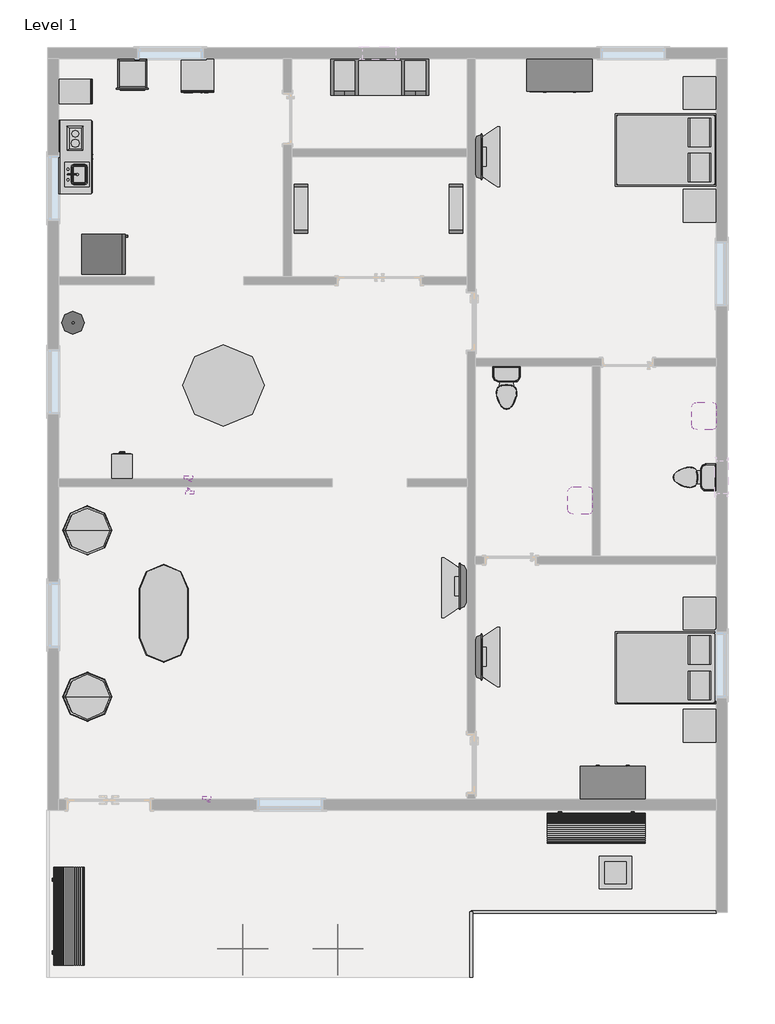
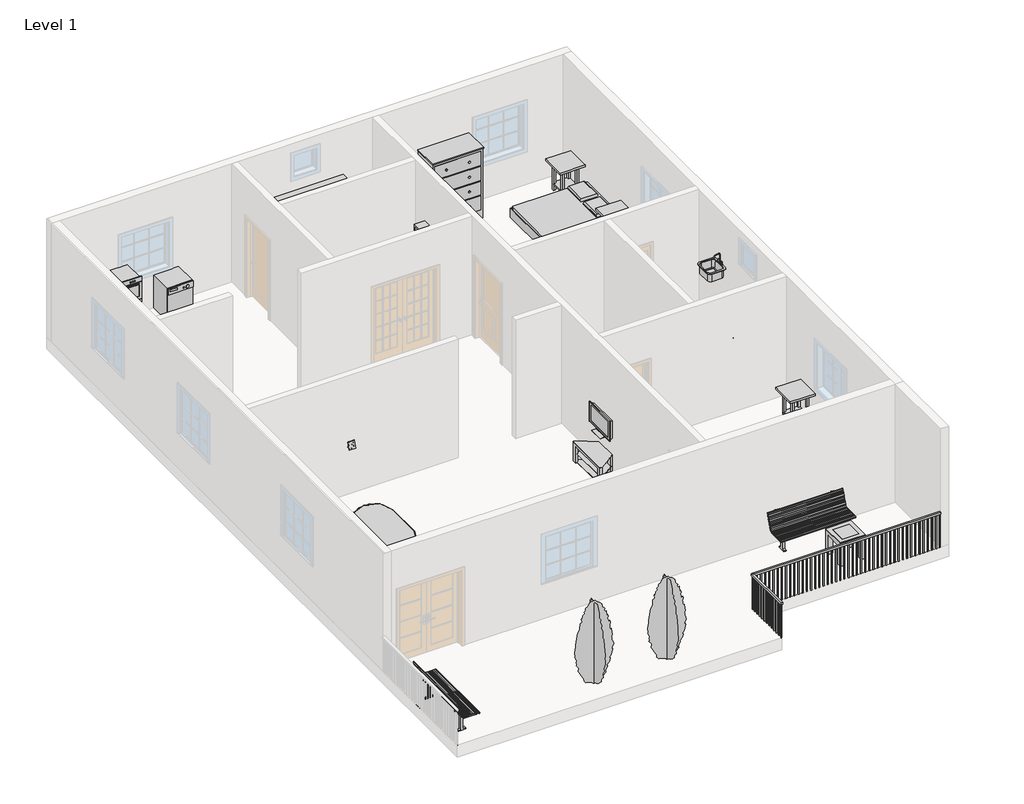
# One storey, part 2 of 2: 24 furniture elements, 11 proxies, 6 flow terminals, 4 geographic elements, 2 railings.
"""IFC4 building model written with IfcOpenShell, lengths in millimetres."""

from ifc_helpers import new_model, si_unit, frame, origin, origin_with_axes, place, context, project, spatial, polyline, outline, extrude, triangles, transform, mapped, element, save
from components import proxy_7e1014cc, proxy_fe84b772, proxy_45b28599, proxy_844211aa, proxy_8b8c2dc4, rpc_picture_frame_rpc_picture_frame_c25e3fe9, proxy_a13a33b2, flow_terminal_871c2e40, flow_terminal_d49f872f, flow_terminal_62a433f7, toilet_domestic_3d_toilet_domestic_3d_f7549cf7, toilet_domestic_3d_toilet_domestic_3d_183bbd19, furniture_c8abb964, furniture_552c1472, furniture_95afb093, furniture_9fa109b2, furniture_cf0b6580, furniture_417d203a, furniture_56245f3a, tv_stand_tv_stand_6ce107e5, furniture_b5c51a22, furniture_2c34a4f9, furniture_bbcc68ce, furniture_5bc9ed15, furniture_c80d6d9c, geographic_element_235d1464, rpc_tree_conifer_chinese_juniper_7_1b9786cd

model = new_model("IFC4")

# Units and contexts
model_context = context("Model", 3, world=origin())
ifc_project = project(units=[si_unit("LENGTHUNIT", "METRE", prefix="MILLI")], contexts=[model_context])

# Site, building, storey
site = spatial("IfcSite", under=ifc_project)
building = spatial("IfcBuilding", under=site)
storey = spatial("IfcBuildingStorey", under=building, Name="Level 1", Elevation=0.0)

# Proxies
placement = place(None, origin())
element("IfcBuildingElementProxy", 1, Name="Building Element Proxy", at=placement, inside=storey, context=model_context, shape_type="Tessellation", body=[
    triangles([(-15555.8644409, -380.8198874, 0.0), (-15555.8644409, -3505.0197784, 0.0), (-7656.4646347, -3505.0197784, 0.0), (-7656.4646347, -2285.8199238, 0.0), (-7647.9977097, -380.8198874, 0.0)], [[1, 2, 4], [4, 3, 5], [3, 4, 2], [4, 5, 1]], closed=False),
])
element("IfcBuildingElementProxy", 2, Name="Building Element Proxy", at=placement, inside=storey, context=model_context, shape_type="Tessellation", body=[
    triangles([(-7656.4646347, -2285.8199238, 0.0), (-3084.4649254, -2285.8199238, 0.0), (-3084.4649254, -380.8198874, 0.0), (-7643.7130875, -380.8198874, 0.0), (-7647.8139999, -380.8198874, 0.0)], [[5, 1, 4], [4, 2, 3], [2, 4, 1]], closed=False),
])
proxy_shape = proxy_7e1014cc(model_context)
element("IfcBuildingElementProxy", 3, Name="18\" x 24\" x 34 1/2\"", ObjectType="18\" x 24\" x 34 1/2\"", at=placement, inside=storey, context=model_context, shape_type="MappedRepresentation", body=[
    mapped(proxy_shape, transform((-14781.4152961, 12724.2626366, 0.0), x_axis=(0.0, 1.0, 0.0), y_axis=(-1.0, 0.0, 0.0), z_axis=(0.0, 0.0, 1.0))),
])
proxy_2_shape = proxy_fe84b772(model_context)
element("IfcBuildingElementProxy", 4, Name="Cook Top-2 Unit : 12\" x 18\"", ObjectType="Cook Top-2 Unit : 12\" x 18\"", at=placement, inside=storey, context=model_context, shape_type="MappedRepresentation", body=[
    mapped(proxy_2_shape, transform((-14971.6648609, 12184.3049007, 0.0), x_axis=(-1.0, 0.0, 0.0), y_axis=(0.0, -1.0, 0.0), z_axis=(0.0, 0.0, 1.0))),
])
proxy_3_shape = proxy_45b28599(model_context)
element("IfcBuildingElementProxy", 5, Name="Dishwasher : 24\" x 24\" x 34\"", ObjectType="Dishwasher : 24\" x 24\" x 34\"", at=placement, inside=storey, context=model_context, shape_type="MappedRepresentation", body=[
    mapped(proxy_3_shape, transform((-13144.1823294, 13068.7305403, 0.0), x_axis=(1.0, 0.0, 0.0), y_axis=(0.0, 1.0, 0.0), z_axis=(0.0, 0.0, 1.0))),
])
proxy_4_shape = proxy_844211aa(model_context)
element("IfcBuildingElementProxy", 6, Name="Kitchenette - Small : 54\"", ObjectType="Kitchenette - Small : 54\"", at=placement, inside=storey, context=model_context, shape_type="MappedRepresentation", body=[
    mapped(proxy_4_shape, transform((-15352.6648609, 11792.4424002, 0.0), x_axis=(0.0, 1.0, 0.0), y_axis=(-1.0, 0.0, 0.0), z_axis=(0.0, 0.0, 1.0))),
])
proxy_5_shape = proxy_8b8c2dc4(model_context)
element("IfcBuildingElementProxy", 7, Name="Oven Double-Built-in : 21 1/2\" x 39 1/4\" x 21\"", ObjectType="Oven Double-Built-in : 21 1/2\" x 39 1/4\" x 21\"", at=placement, inside=storey, context=model_context, shape_type="MappedRepresentation", body=[
    mapped(proxy_5_shape, transform((-13945.8899336, 13219.5142461, 0.0), x_axis=(1.0, 0.0, 0.0), y_axis=(0.0, 1.0, 0.0), z_axis=(0.0, 0.0, 1.0))),
])
rpc_picture_frame_rpc_picture_frame_shape = rpc_picture_frame_rpc_picture_frame_c25e3fe9(model_context)
element("IfcBuildingElementProxy", 8, Name="RPC Picture Frame : RPC Picture Frame", ObjectType="RPC Picture Frame : RPC Picture Frame", at=placement, inside=storey, context=model_context, shape_type="MappedRepresentation", body=[
    mapped(rpc_picture_frame_rpc_picture_frame_shape, transform((-12906.6432707, 5575.4801051, 1219.2), x_axis=(1.0, 0.0, 0.0), y_axis=(0.0, 1.0, 0.0), z_axis=(0.0, 0.0, 1.0))),
])
element("IfcBuildingElementProxy", 9, Name="RPC Picture Frame : RPC Picture Frame", ObjectType="RPC Picture Frame : RPC Picture Frame", at=placement, inside=storey, context=model_context, shape_type="MappedRepresentation", body=[
    mapped(rpc_picture_frame_rpc_picture_frame_shape, transform((-12590.3070473, -177.6198949, 1219.2), x_axis=(-1.0000000000000004, 0.0, 0.0), y_axis=(0.0, -1.0000000000000004, 0.0), z_axis=(0.0, 0.0, 1.0))),
])
element("IfcBuildingElementProxy", 10, Name="RPC Picture Frame : RPC Picture Frame", ObjectType="RPC Picture Frame : RPC Picture Frame", at=placement, inside=storey, context=model_context, shape_type="MappedRepresentation", body=[
    mapped(rpc_picture_frame_rpc_picture_frame_shape, transform((-12931.6137427, 5804.0801051, 1219.2), x_axis=(-1.0, 0.0, 0.0), y_axis=(0.0, -1.0, 0.0), z_axis=(0.0, 0.0, 1.0))),
])
proxy_6_shape = proxy_a13a33b2(model_context)
element("IfcBuildingElementProxy", 11, Name="Refrigerator : 30\" x 32\" RH", ObjectType="Refrigerator : 30\" x 32\" RH", at=placement, inside=storey, context=model_context, shape_type="MappedRepresentation", body=[
    mapped(proxy_6_shape, transform((-14531.9273609, 9993.8811336, 0.0), x_axis=(0.0, 1.000000000000001, 0.0), y_axis=(-1.000000000000001, 0.0, 0.0), z_axis=(0.0, 0.0, 1.0))),
])

# Flow terminals
flow_terminal_shape = flow_terminal_871c2e40(model_context)
element("IfcFlowTerminal", 12, ObjectType="Sink Kitchen-Island : 18\" x 18\"", at=placement, inside=storey, context=model_context, shape_type="MappedRepresentation", body=[
    mapped(flow_terminal_shape, transform((-15007.4194598, 11465.2908645, 0.0), x_axis=(0.0, 1.0, 0.0), y_axis=(-1.0, 0.0, 0.0), z_axis=(0.0, 0.0, 1.0))),
])
flow_terminal_2_shape = flow_terminal_d49f872f(model_context)
element("IfcFlowTerminal", 13, ObjectType="Sink Vanity-Round : 19\" x 19\"", at=placement, inside=storey, context=model_context, shape_type="MappedRepresentation", body=[
    mapped(flow_terminal_2_shape, transform((-15003.148195, 8615.7283645, 609.6), x_axis=(0.0, 1.0000000000000009, 0.0), y_axis=(-1.0000000000000009, 0.0, 0.0), z_axis=(0.0, 0.0, 1.0))),
])
flow_terminal_3_shape = flow_terminal_62a433f7(model_context)
element("IfcFlowTerminal", 14, ObjectType="Sink Vanity-Square : 20\" x 18\"", at=placement, inside=storey, context=model_context, shape_type="MappedRepresentation", body=[
    mapped(flow_terminal_3_shape, transform((-3264.610262, 6988.1693456, 914.4), x_axis=(0.0, -1.0, 0.0), y_axis=(1.0, 0.0, 0.0), z_axis=(0.0, 0.0, 1.0))),
])
element("IfcFlowTerminal", 15, ObjectType="Sink Vanity-Square : 20\" x 18\"", at=placement, inside=storey, context=model_context, shape_type="MappedRepresentation", body=[
    mapped(flow_terminal_3_shape, transform((-5576.010262, 5413.3693456, 914.4), x_axis=(0.0, -1.0000000000000002, 0.0), y_axis=(1.0000000000000002, 0.0, 0.0), z_axis=(0.0, 0.0, 1.0))),
])
toilet_domestic_3d_toilet_domestic_3d_shape = toilet_domestic_3d_toilet_domestic_3d_f7549cf7(model_context)
toilet_domestic_3d_toilet_domestic_3d_2_shape = toilet_domestic_3d_toilet_domestic_3d_183bbd19(model_context)
element("IfcFlowTerminal", 16, ObjectType="Toilet-Domestic-3D : Toilet-Domestic-3D", at=placement, inside=storey, context=model_context, shape_type="MappedRepresentation", body=[
    mapped(toilet_domestic_3d_toilet_domestic_3d_shape, transform((-6996.0648609, 7404.8840777, 0.0), x_axis=(1.0, 0.0, 0.0), y_axis=(0.0, 1.0, 0.0), z_axis=(0.0, 0.0, 1.0))),
    mapped(toilet_domestic_3d_toilet_domestic_3d_2_shape, transform((-6996.0648609, 7404.8840777, 0.0), x_axis=(1.0, 0.0, 0.0), y_axis=(0.0, 1.0, 0.0), z_axis=(0.0, 0.0, 1.0))),
])
element("IfcFlowTerminal", 17, ObjectType="Toilet-Domestic-3D : Toilet-Domestic-3D", at=placement, inside=storey, context=model_context, shape_type="MappedRepresentation", body=[
    mapped(toilet_domestic_3d_toilet_domestic_3d_shape, transform((-3579.1608883, 5829.4801051, 0.0), x_axis=(0.0, -1.0000000000000007, 0.0), y_axis=(1.0000000000000007, 0.0, 0.0), z_axis=(0.0, 0.0, 1.0))),
    mapped(toilet_domestic_3d_toilet_domestic_3d_2_shape, transform((-3579.1608883, 5829.4801051, 0.0), x_axis=(0.0, -1.0000000000000007, 0.0), y_axis=(1.0000000000000007, 0.0, 0.0), z_axis=(0.0, 0.0, 1.0))),
])

# Furniture
furniture_shape = furniture_c8abb964(model_context)
element("IfcFurniture", 18, ObjectType="Bed-Box : Double 53\" x 74\"", at=placement, inside=storey, context=model_context, shape_type="MappedRepresentation", body=[
    mapped(furniture_shape, transform((-3789.8353527, 2612.6325641, 0.0), x_axis=(0.0, -1.0, 0.0), y_axis=(1.0, 0.0, 0.0), z_axis=(0.0, 0.0, 1.0))),
])
element("IfcFurniture", 19, ObjectType="Bed-Box : Double 53\" x 74\"", at=placement, inside=storey, context=model_context, shape_type="MappedRepresentation", body=[
    mapped(furniture_shape, transform((-3789.8353527, 12277.3325641, 0.0), x_axis=(0.0, -1.0, 0.0), y_axis=(1.0, 0.0, 0.0), z_axis=(0.0, 0.0, 1.0))),
])
furniture_2_shape = furniture_552c1472(model_context)
element("IfcFurniture", 20, ObjectType="Cabinet-File 3 Drawer : 15\" x 18\"", at=placement, inside=storey, context=model_context, shape_type="MappedRepresentation", body=[
    mapped(furniture_2_shape, transform((-14299.4613079, 5890.545805, 0.0), x_axis=(-1.0, 0.0, 0.0), y_axis=(0.0, -1.0, 0.0), z_axis=(0.0, 0.0, 1.0))),
])
furniture_3_shape = furniture_95afb093(model_context)
element("IfcFurniture", 21, ObjectType="Counter Top w Sink Hole : 24\" Depth", at=placement, inside=storey, context=model_context, shape_type="MappedRepresentation", body=[
    mapped(furniture_3_shape, transform((-15352.6648609, 12325.8424002, 0.0), x_axis=(0.0, 1.0, 0.0), y_axis=(-1.0, 0.0, 0.0), z_axis=(0.0, 0.0, 1.0))),
])
furniture_4_shape = furniture_9fa109b2(model_context)
element("IfcFurniture", 22, ObjectType="Dresser : 48\" x 72\" x 24\"", at=placement, inside=storey, context=model_context, shape_type="MappedRepresentation", body=[
    mapped(furniture_4_shape, transform((-5284.0581207, -235.982849, 0.0), x_axis=(-1.0000000000000004, 0.0, 0.0), y_axis=(0.0, -1.0000000000000004, 0.0), z_axis=(0.0, 0.0, 1.0))),
])
element("IfcFurniture", 23, ObjectType="Dresser : 48\" x 72\" x 24\"", at=placement, inside=storey, context=model_context, shape_type="MappedRepresentation", body=[
    mapped(furniture_4_shape, transform((-5736.2716011, 13698.3430592, 0.0), x_axis=(1.0, 0.0, 0.0), y_axis=(0.0, 1.0, 0.0), z_axis=(0.0, 0.0, 1.0))),
])
furniture_5_shape = furniture_cf0b6580(model_context)
element("IfcFurniture", 24, ObjectType="Entertainment Center : 72\" x 72\" x 24\"", at=placement, inside=storey, context=model_context, shape_type="MappedRepresentation", body=[
    mapped(furniture_5_shape, transform((-9358.2648609, 13741.5801051, 0.0), x_axis=(1.0, 0.0, 0.0), y_axis=(0.0, 1.0, 0.0), z_axis=(0.0, 0.0, 1.0))),
])
furniture_6_shape = furniture_417d203a(model_context)
element("IfcFurniture", 25, ObjectType="Shelving : 36\" x 10\" x 72\"", at=placement, inside=storey, context=model_context, shape_type="MappedRepresentation", body=[
    mapped(furniture_6_shape, transform((-11136.2648609, 10845.9801051, 0.0), x_axis=(0.0, 1.0000000000000002, 0.0), y_axis=(-1.0000000000000002, 0.0, 0.0), z_axis=(0.0, 0.0, 1.0))),
])
element("IfcFurniture", 26, ObjectType="Shelving : 36\" x 10\" x 72\"", at=placement, inside=storey, context=model_context, shape_type="MappedRepresentation", body=[
    mapped(furniture_6_shape, transform((-8240.6648609, 10845.9801051, 0.0), x_axis=(0.0, 1.0000000000000002, 0.0), y_axis=(-1.0000000000000002, 0.0, 0.0), z_axis=(0.0, 0.0, 1.0))),
])
furniture_7_shape = furniture_56245f3a(model_context)
element("IfcFurniture", 27, ObjectType="TV - Flat Screen : 32\"", at=placement, inside=storey, context=model_context, shape_type="MappedRepresentation", body=[
    mapped(furniture_7_shape, transform((-7521.7262373, 2480.6246192, 914.4), x_axis=(0.0, 1.0000000000000002, 0.0), y_axis=(-1.0000000000000002, 0.0, 0.0), z_axis=(0.0, 0.0, 1.0))),
])
element("IfcFurniture", 28, ObjectType="TV - Flat Screen : 32\"", at=placement, inside=storey, context=model_context, shape_type="MappedRepresentation", body=[
    mapped(furniture_7_shape, transform((-7521.7262373, 11815.1246192, 914.4), x_axis=(0.0, 1.0000000000000002, 0.0), y_axis=(-1.0000000000000002, 0.0, 0.0), z_axis=(0.0, 0.0, 1.0))),
])
element("IfcFurniture", 29, ObjectType="TV - Flat Screen : 32\"", at=placement, inside=storey, context=model_context, shape_type="MappedRepresentation", body=[
    mapped(furniture_7_shape, transform((-7810.4777417, 3791.9647442, 914.4), x_axis=(0.0, -1.0000000000000007, 0.0), y_axis=(1.0000000000000007, 0.0, 0.0), z_axis=(0.0, 0.0, 1.0))),
])
tv_stand_tv_stand_shape = tv_stand_tv_stand_6ce107e5(model_context)
element("IfcFurniture", 30, ObjectType="TV Stand : TV Stand", at=placement, inside=storey, context=model_context, shape_type="MappedRepresentation", body=[
    mapped(tv_stand_tv_stand_shape, transform((-7580.2648609, 11685.992103, 0.0), x_axis=(0.0, 1.0000000000000002, 0.0), y_axis=(-1.0000000000000002, 0.0, 0.0), z_axis=(0.0, 0.0, 1.0))),
])
element("IfcFurniture", 31, ObjectType="TV Stand : TV Stand", at=placement, inside=storey, context=model_context, shape_type="MappedRepresentation", body=[
    mapped(tv_stand_tv_stand_shape, transform((-7580.2648609, 2351.492103, 0.0), x_axis=(0.0, 1.0000000000000002, 0.0), y_axis=(-1.0000000000000002, 0.0, 0.0), z_axis=(0.0, 0.0, 1.0))),
])
element("IfcFurniture", 32, ObjectType="TV Stand : TV Stand", at=placement, inside=storey, context=model_context, shape_type="MappedRepresentation", body=[
    mapped(tv_stand_tv_stand_shape, transform((-7747.8095547, 3895.3169532, 0.0), x_axis=(0.0, -1.0000000000000007, 0.0), y_axis=(1.0000000000000007, 0.0, 0.0), z_axis=(0.0, 0.0, 1.0))),
])
furniture_8_shape = furniture_b5c51a22(model_context)
element("IfcFurniture", 33, ObjectType="Table-Coffee : 24\" x 24\" x 24\"", at=placement, inside=storey, context=model_context, shape_type="MappedRepresentation", body=[
    mapped(furniture_8_shape, transform((-4982.3306276, -1644.4309727, 0.0), x_axis=(1.0, 0.0, 0.0), y_axis=(0.0, 1.0, 0.0), z_axis=(0.0, 0.0, 1.0))),
])
furniture_9_shape = furniture_2c34a4f9(model_context)
element("IfcFurniture", 34, ObjectType="Table-Dining Oval : 36\" x 72\"", at=placement, inside=storey, context=model_context, shape_type="MappedRepresentation", body=[
    mapped(furniture_9_shape, transform((-13754.9632216, 3691.2997772, 0.0), x_axis=(0.0, 1.0000000000000002, 0.0), y_axis=(-1.0000000000000002, 0.0, 0.0), z_axis=(0.0, 0.0, 1.0))),
])
furniture_10_shape = furniture_bbcc68ce(model_context)
element("IfcFurniture", 35, ObjectType="Table-Dining Round w Chairs : 60\" Diameter", at=placement, inside=storey, context=model_context, shape_type="MappedRepresentation", body=[
    mapped(furniture_10_shape, transform((-12382.9468281, 7728.8587936, 0.0), x_axis=(1.0, 0.0, 0.0), y_axis=(0.0, 1.0, 0.0), z_axis=(0.0, 0.0, 1.0))),
])
furniture_11_shape = furniture_5bc9ed15(model_context)
element("IfcFurniture", 36, ObjectType="Table-Night Stand : 24\" x 24\" x 30\"", at=placement, inside=storey, context=model_context, shape_type="MappedRepresentation", body=[
    mapped(furniture_11_shape, transform((-3697.7984912, 2984.6801051, 0.0), x_axis=(1.0, 0.0, 0.0), y_axis=(0.0, 1.0, 0.0), z_axis=(0.0, 0.0, 1.0))),
])
element("IfcFurniture", 37, ObjectType="Table-Night Stand : 24\" x 24\" x 30\"", at=placement, inside=storey, context=model_context, shape_type="MappedRepresentation", body=[
    mapped(furniture_11_shape, transform((-3697.7984912, 889.1801051, 0.0), x_axis=(1.0, 0.0, 0.0), y_axis=(0.0, 1.0, 0.0), z_axis=(0.0, 0.0, 1.0))),
])
element("IfcFurniture", 38, ObjectType="Table-Night Stand : 24\" x 24\" x 30\"", at=placement, inside=storey, context=model_context, shape_type="MappedRepresentation", body=[
    mapped(furniture_11_shape, transform((-3697.7984912, 12700.1801051, 0.0), x_axis=(1.0, 0.0, 0.0), y_axis=(0.0, 1.0, 0.0), z_axis=(0.0, 0.0, 1.0))),
])
element("IfcFurniture", 39, ObjectType="Table-Night Stand : 24\" x 24\" x 30\"", at=placement, inside=storey, context=model_context, shape_type="MappedRepresentation", body=[
    mapped(furniture_11_shape, transform((-3697.7984912, 10591.9801051, 0.0), x_axis=(1.0, 0.0, 0.0), y_axis=(0.0, 1.0, 0.0), z_axis=(0.0, 0.0, 1.0))),
])
furniture_12_shape = furniture_c80d6d9c(model_context)
element("IfcFurniture", 40, ObjectType="Table-Round : 36\" Diameter", at=placement, inside=storey, context=model_context, shape_type="MappedRepresentation", body=[
    mapped(furniture_12_shape, transform((-14819.2648609, 4838.8801051, 0.0), x_axis=(1.0, 0.0, 0.0), y_axis=(0.0, 1.0, 0.0), z_axis=(0.0, 0.0, 1.0))),
])
element("IfcFurniture", 41, ObjectType="Table-Round : 36\" Diameter", at=placement, inside=storey, context=model_context, shape_type="MappedRepresentation", body=[
    mapped(furniture_12_shape, transform((-14819.2648609, 1733.7301051, 0.0), x_axis=(1.0, 0.0, 0.0), y_axis=(0.0, 1.0, 0.0), z_axis=(0.0, 0.0, 1.0))),
])

# Geographic elements
geographic_element_shape = geographic_element_235d1464(model_context)
element("IfcGeographicElement", 42, ObjectType="Park Bench : 72\"", at=placement, inside=storey, context=model_context, shape_type="MappedRepresentation", body=[
    mapped(geographic_element_shape, transform((-15200.2648609, -2362.0198949, 0.0), x_axis=(0.0, 1.0000000000000002, 0.0), y_axis=(-1.0000000000000002, 0.0, 0.0), z_axis=(0.0, 0.0, 1.0))),
])
element("IfcGeographicElement", 43, ObjectType="Park Bench : 72\"", at=placement, inside=storey, context=model_context, shape_type="MappedRepresentation", body=[
    mapped(geographic_element_shape, transform((-5319.6648609, -685.6198949, 0.0), x_axis=(1.0, 0.0, 0.0), y_axis=(0.0, 1.0, 0.0), z_axis=(0.0, 0.0, 1.0))),
])
rpc_tree_conifer_chinese_juniper_7_shape = rpc_tree_conifer_chinese_juniper_7_1b9786cd(model_context)
element("IfcGeographicElement", 44, ObjectType="RPC Tree - Conifer : Chinese Juniper - 7'", at=placement, inside=storey, context=model_context, shape_type="MappedRepresentation", body=[
    mapped(rpc_tree_conifer_chinese_juniper_7_shape, transform((-11923.861532, -2971.6198949, 0.0), x_axis=(1.0, 0.0, 0.0), y_axis=(0.0, 1.0, 0.0), z_axis=(0.0, 0.0, 1.0))),
])
element("IfcGeographicElement", 45, ObjectType="RPC Tree - Conifer : Chinese Juniper - 7'", at=placement, inside=storey, context=model_context, shape_type="MappedRepresentation", body=[
    mapped(rpc_tree_conifer_chinese_juniper_7_shape, transform((-10145.861532, -2971.6198949, 0.0), x_axis=(1.0, 0.0, 0.0), y_axis=(0.0, 1.0, 0.0), z_axis=(0.0, 0.0, 1.0))),
])

# Railings
element("IfcRailing", 46, ObjectType="Handrail - Rectangular", at=placement, inside=storey, context=model_context, shape_type="SweptSolid", body=[
    extrude(outline(polyline([(-3084.4648609, -2260.4198949), (-3084.4648609, -2311.2198949), (-7656.4648609, -2311.2198949), (-7656.4648609, -2260.4198949), (-3084.4648609, -2260.4198949)])), frame((0.0, 0.0, 863.6), z_axis=(0.0, 0.0, 1.0), x_axis=(1.0, 0.0, 0.0)), (0.0, 0.0, 1.0), 50.8),
    extrude(outline(polyline([(-7545.3398609, -2276.2948949), (-7545.3398609, -2295.3448949), (-7564.3898609, -2295.3448949), (-7564.3898609, -2276.2948949), (-7545.3398609, -2276.2948949)])), origin_with_axes(), (0.0, 0.0, 1.0), 863.6),
    extrude(outline(polyline([(-7443.7398609, -2276.2948949), (-7443.7398609, -2295.3448949), (-7462.7898609, -2295.3448949), (-7462.7898609, -2276.2948949), (-7443.7398609, -2276.2948949)])), origin_with_axes(), (0.0, 0.0, 1.0), 863.6),
    extrude(outline(polyline([(-7342.1398609, -2276.2948949), (-7342.1398609, -2295.3448949), (-7361.1898609, -2295.3448949), (-7361.1898609, -2276.2948949), (-7342.1398609, -2276.2948949)])), origin_with_axes(), (0.0, 0.0, 1.0), 863.6),
    extrude(outline(polyline([(-7240.5398609, -2276.2948949), (-7240.5398609, -2295.3448949), (-7259.5898609, -2295.3448949), (-7259.5898609, -2276.2948949), (-7240.5398609, -2276.2948949)])), origin_with_axes(), (0.0, 0.0, 1.0), 863.6),
    extrude(outline(polyline([(-7138.9398609, -2276.2948949), (-7138.9398609, -2295.3448949), (-7157.9898609, -2295.3448949), (-7157.9898609, -2276.2948949), (-7138.9398609, -2276.2948949)])), origin_with_axes(), (0.0, 0.0, 1.0), 863.6),
    extrude(outline(polyline([(-7037.3398609, -2276.2948949), (-7037.3398609, -2295.3448949), (-7056.3898609, -2295.3448949), (-7056.3898609, -2276.2948949), (-7037.3398609, -2276.2948949)])), origin_with_axes(), (0.0, 0.0, 1.0), 863.6),
    extrude(outline(polyline([(-6935.7398609, -2276.2948949), (-6935.7398609, -2295.3448949), (-6954.7898609, -2295.3448949), (-6954.7898609, -2276.2948949), (-6935.7398609, -2276.2948949)])), origin_with_axes(), (0.0, 0.0, 1.0), 863.6),
    extrude(outline(polyline([(-6834.1398609, -2276.2948949), (-6834.1398609, -2295.3448949), (-6853.1898609, -2295.3448949), (-6853.1898609, -2276.2948949), (-6834.1398609, -2276.2948949)])), origin_with_axes(), (0.0, 0.0, 1.0), 863.6),
    extrude(outline(polyline([(-6732.5398609, -2276.2948949), (-6732.5398609, -2295.3448949), (-6751.5898609, -2295.3448949), (-6751.5898609, -2276.2948949), (-6732.5398609, -2276.2948949)])), origin_with_axes(), (0.0, 0.0, 1.0), 863.6),
    extrude(outline(polyline([(-6630.9398609, -2276.2948949), (-6630.9398609, -2295.3448949), (-6649.9898609, -2295.3448949), (-6649.9898609, -2276.2948949), (-6630.9398609, -2276.2948949)])), origin_with_axes(), (0.0, 0.0, 1.0), 863.6),
    extrude(outline(polyline([(-6529.3398609, -2276.2948949), (-6529.3398609, -2295.3448949), (-6548.3898609, -2295.3448949), (-6548.3898609, -2276.2948949), (-6529.3398609, -2276.2948949)])), origin_with_axes(), (0.0, 0.0, 1.0), 863.6),
    extrude(outline(polyline([(-6427.7398609, -2276.2948949), (-6427.7398609, -2295.3448949), (-6446.7898609, -2295.3448949), (-6446.7898609, -2276.2948949), (-6427.7398609, -2276.2948949)])), origin_with_axes(), (0.0, 0.0, 1.0), 863.6),
    extrude(outline(polyline([(-6326.1398609, -2276.2948949), (-6326.1398609, -2295.3448949), (-6345.1898609, -2295.3448949), (-6345.1898609, -2276.2948949), (-6326.1398609, -2276.2948949)])), origin_with_axes(), (0.0, 0.0, 1.0), 863.6),
    extrude(outline(polyline([(-6224.5398609, -2276.2948949), (-6224.5398609, -2295.3448949), (-6243.5898609, -2295.3448949), (-6243.5898609, -2276.2948949), (-6224.5398609, -2276.2948949)])), origin_with_axes(), (0.0, 0.0, 1.0), 863.6),
    extrude(outline(polyline([(-6122.9398609, -2276.2948949), (-6122.9398609, -2295.3448949), (-6141.9898609, -2295.3448949), (-6141.9898609, -2276.2948949), (-6122.9398609, -2276.2948949)])), origin_with_axes(), (0.0, 0.0, 1.0), 863.6),
    extrude(outline(polyline([(-6021.3398609, -2276.2948949), (-6021.3398609, -2295.3448949), (-6040.3898609, -2295.3448949), (-6040.3898609, -2276.2948949), (-6021.3398609, -2276.2948949)])), origin_with_axes(), (0.0, 0.0, 1.0), 863.6),
    extrude(outline(polyline([(-5919.7398609, -2276.2948949), (-5919.7398609, -2295.3448949), (-5938.7898609, -2295.3448949), (-5938.7898609, -2276.2948949), (-5919.7398609, -2276.2948949)])), origin_with_axes(), (0.0, 0.0, 1.0), 863.6),
    extrude(outline(polyline([(-5818.1398609, -2276.2948949), (-5818.1398609, -2295.3448949), (-5837.1898609, -2295.3448949), (-5837.1898609, -2276.2948949), (-5818.1398609, -2276.2948949)])), origin_with_axes(), (0.0, 0.0, 1.0), 863.6),
    extrude(outline(polyline([(-5716.5398609, -2276.2948949), (-5716.5398609, -2295.3448949), (-5735.5898609, -2295.3448949), (-5735.5898609, -2276.2948949), (-5716.5398609, -2276.2948949)])), origin_with_axes(), (0.0, 0.0, 1.0), 863.6),
    extrude(outline(polyline([(-5614.9398609, -2276.2948949), (-5614.9398609, -2295.3448949), (-5633.9898609, -2295.3448949), (-5633.9898609, -2276.2948949), (-5614.9398609, -2276.2948949)])), origin_with_axes(), (0.0, 0.0, 1.0), 863.6),
    extrude(outline(polyline([(-5513.3398609, -2276.2948949), (-5513.3398609, -2295.3448949), (-5532.3898609, -2295.3448949), (-5532.3898609, -2276.2948949), (-5513.3398609, -2276.2948949)])), origin_with_axes(), (0.0, 0.0, 1.0), 863.6),
    extrude(outline(polyline([(-5411.7398609, -2276.2948949), (-5411.7398609, -2295.3448949), (-5430.7898609, -2295.3448949), (-5430.7898609, -2276.2948949), (-5411.7398609, -2276.2948949)])), origin_with_axes(), (0.0, 0.0, 1.0), 863.6),
    extrude(outline(polyline([(-5310.1398609, -2276.2948949), (-5310.1398609, -2295.3448949), (-5329.1898609, -2295.3448949), (-5329.1898609, -2276.2948949), (-5310.1398609, -2276.2948949)])), origin_with_axes(), (0.0, 0.0, 1.0), 863.6),
    extrude(outline(polyline([(-5208.5398609, -2276.2948949), (-5208.5398609, -2295.3448949), (-5227.5898609, -2295.3448949), (-5227.5898609, -2276.2948949), (-5208.5398609, -2276.2948949)])), origin_with_axes(), (0.0, 0.0, 1.0), 863.6),
    extrude(outline(polyline([(-5106.9398609, -2276.2948949), (-5106.9398609, -2295.3448949), (-5125.9898609, -2295.3448949), (-5125.9898609, -2276.2948949), (-5106.9398609, -2276.2948949)])), origin_with_axes(), (0.0, 0.0, 1.0), 863.6),
    extrude(outline(polyline([(-5005.3398609, -2276.2948949), (-5005.3398609, -2295.3448949), (-5024.3898609, -2295.3448949), (-5024.3898609, -2276.2948949), (-5005.3398609, -2276.2948949)])), origin_with_axes(), (0.0, 0.0, 1.0), 863.6),
    extrude(outline(polyline([(-4903.7398609, -2276.2948949), (-4903.7398609, -2295.3448949), (-4922.7898609, -2295.3448949), (-4922.7898609, -2276.2948949), (-4903.7398609, -2276.2948949)])), origin_with_axes(), (0.0, 0.0, 1.0), 863.6),
    extrude(outline(polyline([(-4802.1398609, -2276.2948949), (-4802.1398609, -2295.3448949), (-4821.1898609, -2295.3448949), (-4821.1898609, -2276.2948949), (-4802.1398609, -2276.2948949)])), origin_with_axes(), (0.0, 0.0, 1.0), 863.6),
    extrude(outline(polyline([(-4700.5398609, -2276.2948949), (-4700.5398609, -2295.3448949), (-4719.5898609, -2295.3448949), (-4719.5898609, -2276.2948949), (-4700.5398609, -2276.2948949)])), origin_with_axes(), (0.0, 0.0, 1.0), 863.6),
    extrude(outline(polyline([(-4598.9398609, -2276.2948949), (-4598.9398609, -2295.3448949), (-4617.9898609, -2295.3448949), (-4617.9898609, -2276.2948949), (-4598.9398609, -2276.2948949)])), origin_with_axes(), (0.0, 0.0, 1.0), 863.6),
    extrude(outline(polyline([(-4497.3398609, -2276.2948949), (-4497.3398609, -2295.3448949), (-4516.3898609, -2295.3448949), (-4516.3898609, -2276.2948949), (-4497.3398609, -2276.2948949)])), origin_with_axes(), (0.0, 0.0, 1.0), 863.6),
    extrude(outline(polyline([(-4395.7398609, -2276.2948949), (-4395.7398609, -2295.3448949), (-4414.7898609, -2295.3448949), (-4414.7898609, -2276.2948949), (-4395.7398609, -2276.2948949)])), origin_with_axes(), (0.0, 0.0, 1.0), 863.6),
    extrude(outline(polyline([(-4294.1398609, -2276.2948949), (-4294.1398609, -2295.3448949), (-4313.1898609, -2295.3448949), (-4313.1898609, -2276.2948949), (-4294.1398609, -2276.2948949)])), origin_with_axes(), (0.0, 0.0, 1.0), 863.6),
    extrude(outline(polyline([(-4192.5398609, -2276.2948949), (-4192.5398609, -2295.3448949), (-4211.5898609, -2295.3448949), (-4211.5898609, -2276.2948949), (-4192.5398609, -2276.2948949)])), origin_with_axes(), (0.0, 0.0, 1.0), 863.6),
    extrude(outline(polyline([(-4090.9398609, -2276.2948949), (-4090.9398609, -2295.3448949), (-4109.9898609, -2295.3448949), (-4109.9898609, -2276.2948949), (-4090.9398609, -2276.2948949)])), origin_with_axes(), (0.0, 0.0, 1.0), 863.6),
    extrude(outline(polyline([(-3989.3398609, -2276.2948949), (-3989.3398609, -2295.3448949), (-4008.3898609, -2295.3448949), (-4008.3898609, -2276.2948949), (-3989.3398609, -2276.2948949)])), origin_with_axes(), (0.0, 0.0, 1.0), 863.6),
    extrude(outline(polyline([(-3887.7398609, -2276.2948949), (-3887.7398609, -2295.3448949), (-3906.7898609, -2295.3448949), (-3906.7898609, -2276.2948949), (-3887.7398609, -2276.2948949)])), origin_with_axes(), (0.0, 0.0, 1.0), 863.6),
    extrude(outline(polyline([(-3786.1398609, -2276.2948949), (-3786.1398609, -2295.3448949), (-3805.1898609, -2295.3448949), (-3805.1898609, -2276.2948949), (-3786.1398609, -2276.2948949)])), origin_with_axes(), (0.0, 0.0, 1.0), 863.6),
    extrude(outline(polyline([(-3684.5398609, -2276.2948949), (-3684.5398609, -2295.3448949), (-3703.5898609, -2295.3448949), (-3703.5898609, -2276.2948949), (-3684.5398609, -2276.2948949)])), origin_with_axes(), (0.0, 0.0, 1.0), 863.6),
    extrude(outline(polyline([(-3582.9398609, -2276.2948949), (-3582.9398609, -2295.3448949), (-3601.9898609, -2295.3448949), (-3601.9898609, -2276.2948949), (-3582.9398609, -2276.2948949)])), origin_with_axes(), (0.0, 0.0, 1.0), 863.6),
    extrude(outline(polyline([(-3481.3398609, -2276.2948949), (-3481.3398609, -2295.3448949), (-3500.3898609, -2295.3448949), (-3500.3898609, -2276.2948949), (-3481.3398609, -2276.2948949)])), origin_with_axes(), (0.0, 0.0, 1.0), 863.6),
    extrude(outline(polyline([(-3379.7398609, -2276.2948949), (-3379.7398609, -2295.3448949), (-3398.7898609, -2295.3448949), (-3398.7898609, -2276.2948949), (-3379.7398609, -2276.2948949)])), origin_with_axes(), (0.0, 0.0, 1.0), 863.6),
    extrude(outline(polyline([(-3278.1398609, -2276.2948949), (-3278.1398609, -2295.3448949), (-3297.1898609, -2295.3448949), (-3297.1898609, -2276.2948949), (-3278.1398609, -2276.2948949)])), origin_with_axes(), (0.0, 0.0, 1.0), 863.6),
    extrude(outline(polyline([(-3176.5398609, -2276.2948949), (-3176.5398609, -2295.3448949), (-3195.5898609, -2295.3448949), (-3195.5898609, -2276.2948949), (-3176.5398609, -2276.2948949)])), origin_with_axes(), (0.0, 0.0, 1.0), 863.6),
    extrude(outline(polyline([(-7637.4148609, -2276.2948949), (-7637.4148609, -2295.3448949), (-7656.4648609, -2295.3448949), (-7656.4648609, -2276.2948949), (-7637.4148609, -2276.2948949)])), origin_with_axes(), (0.0, 0.0, 1.0), 863.6),
    extrude(outline(polyline([(-3084.4648609, -2276.2948949), (-3084.4648609, -2295.3448949), (-3103.5148609, -2295.3448949), (-3103.5148609, -2276.2948949), (-3084.4648609, -2276.2948949)])), origin_with_axes(), (0.0, 0.0, 1.0), 863.6),
])
element("IfcRailing", 47, ObjectType="Handrail - Rectangular", at=placement, inside=storey, context=model_context, shape_type="SweptSolid", body=[
    extrude(outline(polyline([(-7681.8648609, -2276.2948949), (-7631.0648609, -2276.2948949), (-7631.0648609, -3505.0198949), (-7681.8648609, -3505.0198949), (-7681.8648609, -2276.2948949)])), frame((0.0, 0.0, 863.6), z_axis=(0.0, 0.0, 1.0), x_axis=(1.0, 0.0, 0.0)), (0.0, 0.0, 1.0), 50.8),
    extrude(outline(polyline([(-7665.9898609, -3485.9698949), (-7646.9398609, -3485.9698949), (-7646.9398609, -3505.0198949), (-7665.9898609, -3505.0198949), (-7665.9898609, -3485.9698949)])), origin_with_axes(), (0.0, 0.0, 1.0), 863.6),
    extrude(outline(polyline([(-7665.9898609, -3384.3698949), (-7646.9398609, -3384.3698949), (-7646.9398609, -3403.4198949), (-7665.9898609, -3403.4198949), (-7665.9898609, -3384.3698949)])), origin_with_axes(), (0.0, 0.0, 1.0), 863.6),
    extrude(outline(polyline([(-7665.9898609, -3282.7698949), (-7646.9398609, -3282.7698949), (-7646.9398609, -3301.8198949), (-7665.9898609, -3301.8198949), (-7665.9898609, -3282.7698949)])), origin_with_axes(), (0.0, 0.0, 1.0), 863.6),
    extrude(outline(polyline([(-7665.9898609, -3181.1698949), (-7646.9398609, -3181.1698949), (-7646.9398609, -3200.2198949), (-7665.9898609, -3200.2198949), (-7665.9898609, -3181.1698949)])), origin_with_axes(), (0.0, 0.0, 1.0), 863.6),
    extrude(outline(polyline([(-7665.9898609, -3079.5698949), (-7646.9398609, -3079.5698949), (-7646.9398609, -3098.6198949), (-7665.9898609, -3098.6198949), (-7665.9898609, -3079.5698949)])), origin_with_axes(), (0.0, 0.0, 1.0), 863.6),
    extrude(outline(polyline([(-7665.9898609, -2977.9698949), (-7646.9398609, -2977.9698949), (-7646.9398609, -2997.0198949), (-7665.9898609, -2997.0198949), (-7665.9898609, -2977.9698949)])), origin_with_axes(), (0.0, 0.0, 1.0), 863.6),
    extrude(outline(polyline([(-7665.9898609, -2876.3698949), (-7646.9398609, -2876.3698949), (-7646.9398609, -2895.4198949), (-7665.9898609, -2895.4198949), (-7665.9898609, -2876.3698949)])), origin_with_axes(), (0.0, 0.0, 1.0), 863.6),
    extrude(outline(polyline([(-7665.9898609, -2774.7698949), (-7646.9398609, -2774.7698949), (-7646.9398609, -2793.8198949), (-7665.9898609, -2793.8198949), (-7665.9898609, -2774.7698949)])), origin_with_axes(), (0.0, 0.0, 1.0), 863.6),
    extrude(outline(polyline([(-7665.9898609, -2673.1698949), (-7646.9398609, -2673.1698949), (-7646.9398609, -2692.2198949), (-7665.9898609, -2692.2198949), (-7665.9898609, -2673.1698949)])), origin_with_axes(), (0.0, 0.0, 1.0), 863.6),
    extrude(outline(polyline([(-7665.9898609, -2571.5698949), (-7646.9398609, -2571.5698949), (-7646.9398609, -2590.6198949), (-7665.9898609, -2590.6198949), (-7665.9898609, -2571.5698949)])), origin_with_axes(), (0.0, 0.0, 1.0), 863.6),
    extrude(outline(polyline([(-7665.9898609, -2469.9698949), (-7646.9398609, -2469.9698949), (-7646.9398609, -2489.0198949), (-7665.9898609, -2489.0198949), (-7665.9898609, -2469.9698949)])), origin_with_axes(), (0.0, 0.0, 1.0), 863.6),
    extrude(outline(polyline([(-7665.9898609, -2368.3698949), (-7646.9398609, -2368.3698949), (-7646.9398609, -2387.4198949), (-7665.9898609, -2387.4198949), (-7665.9898609, -2368.3698949)])), origin_with_axes(), (0.0, 0.0, 1.0), 863.6),
    extrude(outline(polyline([(-7665.9898609, -3485.9698949), (-7646.9398609, -3485.9698949), (-7646.9398609, -3505.0198949), (-7665.9898609, -3505.0198949), (-7665.9898609, -3485.9698949)])), origin_with_axes(), (0.0, 0.0, 1.0), 863.6),
    extrude(outline(polyline([(-7665.9898609, -2276.2948949), (-7646.9398609, -2276.2948949), (-7646.9398609, -2295.3448949), (-7665.9898609, -2295.3448949), (-7665.9898609, -2276.2948949)])), origin_with_axes(), (0.0, 0.0, 1.0), 863.6),
])

save(model, "model.ifc")

# Revit data of these elements
# Type "18\" x 24\" x 34 1/2\""
#   Label = "T"
#   Assembly Code = "E1090400"
#   Depth = 2' - 0"
#   Height = 2' - 10 1/2"
#   Width = 1' - 6"
#   Panel Face Material = Plastic, Opaque Black
#   Trach Compact. Material = Steel, Paint Finish, Ivory, Matte
#   Default Elevation = 0
# Type "Cook Top-2 Unit : 12\" x 18\""
#   Assembly Code = "E1090400"
#   Counter Height = 3' - 0"
#   Depth = 1' - 6"
#   Width = 1' - 0"
#   Burner Material = Steel, Chrome Plated
#   Cooktop Material = Steel, Polished
#   Default Elevation = 0
# Type "Dishwasher : 24\" x 24\" x 34\""
#   Label = "DW"
#   Assembly Code = "E1090400"
#   Depth = 2' - 0"
#   Height = 2' - 10"
#   Width = 2' - 0"
#   Dishwasher Material = Steel, Paint Finish, Ivory, Glossy
#   Panel Face Material = Plastic, Opaque Black
#   Default Elevation = 0
# Type "Kitchenette - Small : 54\""
#   Assembly Code = "E1090400"
#   Width = 4' - 6"
#   Height = 2' - 10 1/2"
#   Depth = 2' - 0"
#   Toe Depth = 0' - 3"
#   Toe Height = 0' - 3 1/2"
#   Cabinet Material = Cabinets
#   Door/Drawer Material = Cabinets
#   Handle Material = Cabinets - Handles
#   Default Elevation = 0
# Type "Oven Double-Built-in : 21 1/2\" x 39 1/4\" x 21\""
#   Label = "OVEN"
#   Assembly Code = "E1090400"
#   Depth = 1' - 9"
#   Height = 3' - 3 1/4"
#   Width = 1' - 9 1/2"
#   Oven Material = Metal - Stainless Steel, Polished
#   Default Elevation = 0
# Type "RPC Picture Frame : RPC Picture Frame"
#   built-in parameter 1005198 = "{2, 15},{39, RPC-16-8M5E-0H3T-F0AH-3U0K-JLQ7-G28B-AU},{1, 0},{1, 0},{2, 19},{1, 8},{5, Color},{1, 0},{1, 0},{3, 0.8},{3, 0.8},{3, 0.8},{1, 8},{7, BBoxMin},{1, 0},{1, 0},{1, 0},{1, 0},{1, 0},{1, 8},{7, BBoxMax},{1, 0},{1, 0},{1, 0},{1, 0},{1, 0},{2, 11},{9, RPCTypeId},{1, 0},{1, 0},{39, RPC-16-8M5E-0H3T-F0AH-3U0K-JLQ7-G28B-AU},{1, 6},{14, RPCPlantHeight},{1, 0},{1, 0},{5, 0.625},{2, 11},{7, keyword},{1, 0},{1, 0},{33, :RPCs:Office Clutter:Geometry:RPC},{2, 11},{8, category},{1, 0},{1, 0},{14, Office Clutter},{2, 11},{12, LocalizedUID},{1, 0},{1, 0},{13, Picture Frame},{2, 14},{6, Height},{1, 0},{1, 0},{5, 0.625},{1, 2},{16, Cast Reflections},{1, 0},{1, 0},{1, 0},{1, 2},{8, Portrait},{1, 0},{1, 0},{1, 1},{1, 2},{5, Stand},{1, 0},{1, 0},{1, 1},{2, 11},{10, RPCL_Frame},{1, 0},{1, 0},{5, Frame},{1, 4},{14, Frame Material},{1, 0},{1, 0},{1, 0},{2, 11},{12, RPCL_Picture},{1, 0},{1, 0},{7, Picture},{2, 11},{15, Picture Preview},{1, 0},{1, 0},{65, __RPC:/object data/textures/object/Photo/Photo0/textures/Portrait},{2, 11},{17, i_Picture Preview},{1, 0},{1, 0},{0, },{1, 2},{18, Use Custom Picture},{1, 0},{1, 0},{1, 0},{2, 11},{17, Picture File Name},{1, 0},{1, 0},{0, },{21, assetlibrary_base.fbx},{1, 5},"
#   built-in parameter 1005195 = "RPC-16-8M5E-0H3T-F0AH-3U0K-JLQ7-G28B-AU"
#   Height = 0
# Type "Refrigerator : 30\" x 32\" RH"
#   Label = "REF."
#   Assembly Code = "E1090400"
#   Depth = 2' - 7 3/4"
#   Handle = 2' - 3"
#   Height = 5' - 10"
#   Rear Clearance = 0' - 2"
#   Top Door Height = 1' - 8"
#   Width = 2' - 5 3/8"
#   Material = Steel, Paint Finish, Ivory, Glossy
#   Default Elevation = 0
# Type "Sink Kitchen-Island : 18\" x 18\""
#   Assembly Code = "D2010410"
#   Counter Height = 3' - 0"
#   Depth = 1' - 6"
#   Width = 1' - 6"
#   Faucet Material = Steel, Polished
#   Sink Material = Steel, Polished
#   Default Elevation = 0
# Type "Sink Vanity-Round : 19\" x 19\""
#   Assembly Code = "D2010400"
#   Top Of Counter = 2' - 7"
#   Basin Material = Porcelain, Linen
#   Faucet Material = Steel, Polished
#   Default Elevation = 0
# Type "Sink Vanity-Square : 20\" x 18\""
#   Assembly Code = "D2010400"
#   Counter Height = 2' - 7"
#   Depth = 1' - 6"
#   Width = 1' - 8"
#   Basin Material = Porcelain, Linen
#   Faucet Material = Steel, Polished
#   Default Elevation = 0
# Type "Toilet-Domestic-3D : Toilet-Domestic-3D"
#   Assembly Code = "D2010110"
#   Toilet - Bowl/Basin Material = Porcelain, Linen
#   Toilet - Seat Material = Laminate, Linen, Matte
#   Default Elevation = 0
# Type "Bed-Box : Double 53\" x 74\""
#   Assembly Code = "E2020200"
#   Length = 6' - 2"
#   Width = 4' - 5"
#   Frame Material = Birch
#   Mattress Material = Linen, White
#   Default Elevation = 0
# Type "Cabinet-File 3 Drawer : 15\" x 18\""
#   Assembly Code = "E2020200"
#   Depth = 1' - 6"
#   Height = 3' - 5"
#   Width = 1' - 3"
#   Cabinet Material = Steel, Paint Finish, Ivory, Glossy
#   Handle Material = Steel, Chrome Plated
#   Default Elevation = 0
# Type "Counter Top w Sink Hole : 24\" Depth"
#   Assembly Code = "C1030400"
#   Counter Thickness = 0' - 1 1/2"
#   Depth [instance default] = 2' - 1"
#   Height = 3' - 0"
#   Length [instance default] = 8' - 0"
#   Sink Location [instance default] = 2' - 0"
#   Sink Location To Wall [instance default] = 0' - 6"
#   Sink Opening Depth [instance default] = 1' - 3"
#   Sink Opening Width [instance default] = 2' - 3"
#   Counter Top Material = none
#   Default Elevation = 0
# Type "Dresser : 48\" x 72\" x 24\""
#   Assembly Code = "E2020200"
#   Depth = 2' - 0"
#   Height = 6' - 0"
#   Width = 4' - 0"
#   Dresser Material = Laminate - Ivory, Glossy
#   Drawer Material = Laminate, Ivory, Matte
#   Knob Material = Cherry
#   Default Elevation = 0
# Type "Entertainment Center : 72\" x 72\" x 24\""
#   Assembly Code = "E2020200"
#   Center Width = 2' - 8"
#   Depth = 2' - 0"
#   Height = 6' - 0"
#   Width = 6' - 0"
#   Material = none
#   Default Elevation = 0
# Type "Shelving : 36\" x 10\" x 72\""
#   Assembly Code = "E2020200"
#   Depth = 0' - 10"
#   Height = 6' - 0"
#   Width = 3' - 0"
#   Shelving Unit Material = Birch
#   Default Elevation = 0
# Type "TV - Flat Screen : 32\""
#   SinAng = 0' - 0.0193"
#   L = 2' - 3.79372"
#   H = 1' - 3.6354"
#   Thickness = 0' - 4.33071"
#   Diagonal = 2' - 7.88976"
#   CosAng = 0' - 0.03431"
#   Stand [instance default] = yes
#   Default Elevation = 0
# Type "TV Stand : TV Stand"
#   Depth = 1' - 6"
#   Width = 3' - 8"
#   Height = 1' - 7 1/2"
#   Finish = Melamine - Gray
#   Default Elevation = 0
# Type "Table-Coffee : 24\" x 24\" x 24\""
#   Assembly Code = "E2020200"
#   Height = 2' - 0"
#   Length = 2' - 0"
#   Width = 2' - 0"
#   Top Material = none
#   Frame Material = none
#   Default Elevation = 0
# Type "Table-Dining Oval : 36\" x 72\""
#   Assembly Code = "E2020200"
#   Length = 6' - 0"
#   Width = 3' - 0"
#   Base Material = Steel, Chrome Plated
#   Top Material = Glass - Clear, Grey
#   Default Elevation = 0
#   Description = (empty or 0)
# Type "Table-Dining Round w Chairs : 60\" Diameter"
#   Assembly Code = "E2020200"
#   Radius = 2' - 6"
#   Diameter = 5' - 0"
#   Height = 2' - 6"
#   Chairs = 6
#   Base Material = Pine
#   Top Material = Laminate, Linen, Matte
#   Default Elevation = 0
# Type "Table-Night Stand : 24\" x 24\" x 30\""
#   Assembly Code = "E2020200"
#   Depth = 2' - 0"
#   Height = 2' - 6"
#   Width = 2' - 0"
#   Base Material = Birch
#   Top Material = Laminate, Ivory, Matte
#   Default Elevation = 0
# Type "Table-Round : 36\" Diameter"
#   Assembly Code = "E2020200"
#   Base Radius = 0' - 10"
#   Height = 2' - 6"
#   Radius = 1' - 6"
#   Base Material = Steel, Chrome Plated
#   Top Material = Birch
#   Default Elevation = 0
# Type "Park Bench : 72\""
#   Length = 6' - 0"
#   Seat Material = Wood - Teak
#   Frame Material = Steel, Paint Finish, Dark Gray, Matte
# Type "RPC Tree - Conifer : Chinese Juniper - 7'"
#   built-in parameter 1005198 = "{2, 15},{39, RPC-16-FUM3-UUQ0-UBF0-N000-ST1L-LVER-AU},{1, 0},{1, 0},{2, 13},{1, 8},{5, Color},{1, 0},{1, 0},{3, 0.8},{3, 0.8},{3, 0.8},{1, 8},{7, BBoxMin},{1, 0},{1, 0},{1, 0},{1, 0},{1, 0},{1, 8},{7, BBoxMax},{1, 0},{1, 0},{1, 0},{1, 0},{1, 0},{2, 11},{9, RPCTypeId},{1, 0},{1, 0},{39, RPC-16-FUM3-UUQ0-UBF0-N000-ST1L-LVER-AU},{1, 6},{14, RPCPlantHeight},{1, 0},{1, 0},{1, 7},{2, 11},{7, keyword},{1, 0},{1, 0},{34, :RPCs:Trees [General]:Geometry:RPC},{2, 11},{8, category},{1, 0},{1, 0},{15, Trees [General]},{2, 11},{12, LocalizedUID},{1, 0},{1, 0},{15, Chinese Juniper},{2, 14},{6, Height},{1, 0},{1, 0},{1, 7},{1, 2},{16, Cast Reflections},{1, 0},{1, 0},{1, 0},{1, 2},{12, Cast Shadows},{1, 0},{1, 0},{1, 1},{1, 2},{9, Lock View},{1, 0},{1, 0},{1, 0},{1, 4},{5, ViewC},{1, 0},{1, 0},{1, 0},{21, assetlibrary_base.fbx},{1, 5},"
#   built-in parameter 1005195 = "RPC-16-FUM3-UUQ0-UBF0-N000-ST1L-LVER-AU"
#   Type Comments = "Chinese Juniper"
#   Assembly Code = "G2050500"
#   Height = 7' - 0"
#   Description = (empty or 0)
#   Default Elevation = 0
# Type "Handrail - Rectangular"
#   Assembly Code = "C2010400"
#   built-in parameter 1008612 = 0.0416667 (stored number, unit not read)
#   built-in parameter 1008611 = 0.0416667 (stored number, unit not read)
#   built-in parameter 1008609 = 0.333333 (stored number, unit not read)
#   built-in parameter 1008604 = 0.166667 (stored number, unit not read)
#   built-in parameter 1008603 = 0.166667 (stored number, unit not read)
#   Railing Height = 3' - 0"
#   built-in parameter 1008630 = 2
#   built-in parameter 1008610 = 2
#   built-in parameter 1008618 = Baluster - Square : 3/4"
# Elements 1, 2 (IfcBuildingElementProxy)
#   Material = none
#   Phase Created = New Construction
# Element 3 (IfcBuildingElementProxy, "18\" x 24\" x 34 1/2\"")
#   Phase Created = New Construction
#   Materials on its faces: "Steel, Paint Finish, Ivory, Matte", "Plastic, Opaque Black"
# Element 4 (IfcBuildingElementProxy, "Cook Top-2 Unit : 12\" x 18\"")
#   Phase Created = New Construction
#   Materials on its faces: "Steel, Chrome Plated", "Steel, Polished"
# Element 5 (IfcBuildingElementProxy, "Dishwasher : 24\" x 24\" x 34\"")
#   Phase Created = New Construction
#   Materials on its faces: "Steel, Paint Finish, Ivory, Glossy", "Plastic, Opaque Black"
# Element 6 (IfcBuildingElementProxy, "Kitchenette - Small : 54\"")
#   Phase Created = New Construction
#   Materials on its faces: "Cabinets", "Cabinets - Handles"
# Element 7 (IfcBuildingElementProxy, "Oven Double-Built-in : 21 1/2\" x 39 1/4\" x 21\"")
#   Phase Created = New Construction
#   Materials on its faces: "Steel", "Metal - Stainless Steel, Polished", "Glass"
# Elements 8, 9, 10 (IfcBuildingElementProxy, "RPC Picture Frame : RPC Picture Frame")
#   Phase Created = New Construction
# Element 11 (IfcBuildingElementProxy, "Refrigerator : 30\" x 32\" RH")
#   Phase Created = New Construction
#   Materials on its faces: "Steel, Paint Finish, Ivory, Glossy", "Steel, Chrome Plated"
# Element 12 (IfcFlowTerminal, "Sink Kitchen-Island : 18\" x 18\"")
#   Mark = "7"
#   Phase Created = New Construction
#   Materials on its faces: "Steel, Polished"
# Element 13 (IfcFlowTerminal, "Sink Vanity-Round : 19\" x 19\"")
#   Mark = "8"
#   Phase Created = New Construction
#   Materials on its faces: "Porcelain, Linen", "Steel, Polished"
# Element 14 (IfcFlowTerminal, "Sink Vanity-Square : 20\" x 18\"")
#   Mark = "5"
#   Phase Created = New Construction
#   Materials on its faces: "Porcelain, Linen", "Steel, Polished"
# Element 15 (IfcFlowTerminal, "Sink Vanity-Square : 20\" x 18\"")
#   Mark = "6"
#   Phase Created = New Construction
#   Materials on its faces: "Porcelain, Linen", "Steel, Polished"
# Element 16 (IfcFlowTerminal, "Toilet-Domestic-3D : Toilet-Domestic-3D")
#   Mark = "3"
#   Phase Created = New Construction
#   Materials on its faces: "Porcelain, Linen", "Laminate, Linen, Matte"
# Element 17 (IfcFlowTerminal, "Toilet-Domestic-3D : Toilet-Domestic-3D")
#   Mark = "4"
#   Phase Created = New Construction
#   Materials on its faces: "Porcelain, Linen", "Laminate, Linen, Matte"
# Elements 18, 19 (IfcFurniture, "Bed-Box : Double 53\" x 74\"")
#   Phase Created = New Construction
#   Materials on its faces: "Birch", "Linen, White"
# Element 20 (IfcFurniture, "Cabinet-File 3 Drawer : 15\" x 18\"")
#   Phase Created = New Construction
#   Materials on its faces: "Steel, Chrome Plated", "Steel, Paint Finish, Ivory, Glossy"
# Element 21 (IfcFurniture, "Counter Top w Sink Hole : 24\" Depth")
#   Sink Opening Depth = 1' - 3"
#   Sink Location To Wall = 0' - 6"
#   Length = 4' - 6"
#   Sink Location = 1' - 2"
#   Sink Opening Width = 1' - 4"
#   Depth = 2' - 0"
#   Phase Created = New Construction
#   Materials on its faces: "Counter Top"
# Elements 22, 23 (IfcFurniture, "Dresser : 48\" x 72\" x 24\"")
#   Phase Created = New Construction
#   Materials on its faces: "Laminate, Ivory, Matte", "Cherry", "Laminate - Ivory, Glossy"
# Element 24 (IfcFurniture, "Entertainment Center : 72\" x 72\" x 24\"")
#   Phase Created = New Construction
#   Materials on its faces: "Steel, Chrome Plated", "Glass - Clear, Grey"
# Elements 25, 26 (IfcFurniture, "Shelving : 36\" x 10\" x 72\"")
#   Phase Created = New Construction
#   Materials on its faces: "Birch"
# Elements 27, 28, 29 (IfcFurniture, "TV - Flat Screen : 32\"")
#   Stand = yes
#   Phase Created = New Construction
#   Materials on its faces: "TV - Black", "TV - Glass", "TV - Screen"
# Elements 30, 31, 32 (IfcFurniture, "TV Stand : TV Stand")
#   Phase Created = New Construction
#   Materials on its faces: "Melamine - Gray", "Glass - Shelves"
# Element 33 (IfcFurniture, "Table-Coffee : 24\" x 24\" x 24\"")
#   Phase Created = New Construction
#   Materials on its faces: "Glass - Clear, Grey"
# Element 34 (IfcFurniture, "Table-Dining Oval : 36\" x 72\"")
#   Phase Created = New Construction
#   Materials on its faces: "Steel, Chrome Plated", "Glass - Clear, Grey"
# Element 35 (IfcFurniture, "Table-Dining Round w Chairs : 60\" Diameter")
#   Phase Created = New Construction
#   Materials on its faces: "Pine", "Laminate, Linen, Matte"
# Elements 36, 37, 38, 39 (IfcFurniture, "Table-Night Stand : 24\" x 24\" x 30\"")
#   Phase Created = New Construction
#   Materials on its faces: "Birch", "Laminate, Ivory, Matte"
# Elements 40, 41 (IfcFurniture, "Table-Round : 36\" Diameter")
#   Phase Created = New Construction
#   Materials on its faces: "Steel, Chrome Plated", "Birch"
# Elements 42, 43 (IfcGeographicElement, "Park Bench : 72\"")
#   Phase Created = New Construction
#   Materials on its faces: "Wood - Teak", "Steel, Paint Finish, Dark Gray, Matte"
# Elements 44, 45 (IfcGeographicElement, "RPC Tree - Conifer : Chinese Juniper - 7'")
#   Phase Created = New Construction
# Elements 46, 47 (IfcRailing, "Handrail - Rectangular")
#   Phase Created = New Construction
# Materials
#   "Plastic, Opaque Black": class "Plastic", colour RGB 0 0 0, transparency 0.7, Description = "Plastic, generic, opaque black", Cost = 0
#   "Steel, Paint Finish, Ivory, Matte": class "Metal", colour RGB 247 247 239, transparency 0, Description = "Steel, paint finish, ivory, matte", Cost = 0
#   "Steel, Chrome Plated": class "Metal", colour RGB 17 17 17, transparency 0, Description = "Chromiuim plated steel", Cost = 0
#   "Steel, Polished": class "Metal", colour RGB 57 57 57, transparency 0, Description = "Polished steel", Cost = 0
#   "Steel, Paint Finish, Ivory, Glossy": class "Metal", colour RGB 247 247 239, transparency 0, Description = "Steel, paint finish, ivory, glossy", Cost = 0
#   "Cabinets": colour RGB 249 249 249, transparency 0
#   "Cabinets - Handles": class "Metal", colour RGB 57 57 57, transparency 0
#   "Metal - Stainless Steel, Polished": class "Metal", colour RGB 216 216 216, transparency 0
#   "Porcelain, Linen": class "Ceramic", colour RGB 249 239 230, transparency 0, Description = "Porcelain, linen", Cost = 0
#   "Laminate, Linen, Matte": class "Plastic", colour RGB 249 239 230, transparency 0, Description = "Plastic Laminate - Linen, Matte", Cost = 0
#   "Birch": class "Wood", colour RGB 224 178 126, transparency 0, Description = "Betula Alleghaniensis", Cost = 0
#   "Linen, White": class "Textile", colour RGB 247 247 239, transparency 0, Description = "Linen, white", Cost = 0
#   "Laminate - Ivory, Glossy": colour RGB 247 247 239, transparency 0
#   "Laminate, Ivory, Matte": class "Plastic", colour RGB 247 247 239, transparency 0, Description = "Plastic Laminate - Ivory, Matte", Cost = 0
#   "Cherry": class "Wood", colour RGB 226 177 128, transparency 0, Description = "Prunus Serotina", Cost = 0
#   "Melamine - Gray": class "Wood", colour RGB 49 49 49, transparency 0
#   "Glass - Clear, Grey": class "Glass", colour RGB 252 255 255, transparency 0.64
#   "Pine": class "Wood", colour RGB 223 192 134, transparency 0, Description = "Pinus Echinata", Cost = 0
#   "Wood - Teak": class "Wood", colour RGB 145 112 90, transparency 0
#   "Steel, Paint Finish, Dark Gray, Matte": class "Metal", colour RGB 98 98 98, transparency 0, Description = "Steel, paint finish, dark gray, matte", Cost = 0
#   "Steel": class "Metal", colour RGB 247 247 247, transparency 0, Description = "Steel, mill finish", Cost = 0
#   "Glass": class "Glass", colour RGB 0 128 192, transparency 0.75, Description = "Soda Lime Glass", Cost = 0
#   "Counter Top": class "Wood", colour RGB 226 177 128, transparency 0
#   "TV - Black": colour RGB 49 49 49, transparency 0
#   "TV - Glass": colour RGB 157 157 157, transparency 0.9
#   "TV - Screen": colour RGB 0 0 0, transparency 0
#   "Glass - Shelves": class "Glass", colour RGB 167 167 167, transparency 0.9
